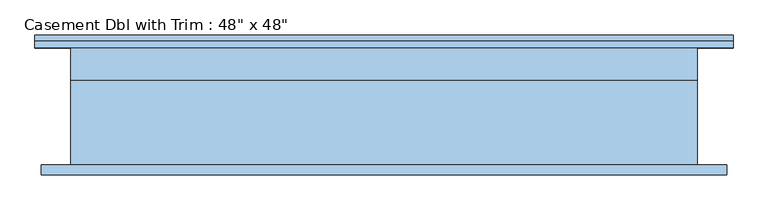
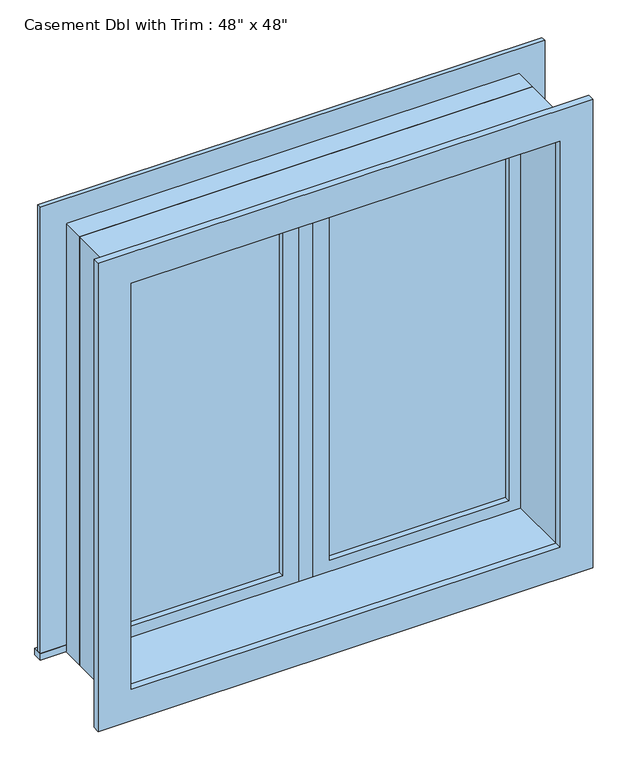
"""IFC4 building model written with IfcOpenShell, lengths in millimetres: window geometry."""

from ifc_helpers import new_model, si_unit, frame, origin, place, context, project, spatial, polyline, outline, extrude, source, transform, mapped, element, save


def window_8af0dca1(model_context):
    return source(origin(), model_context, "Body", "SweptSolid", [
        extrude(outline(polyline([(63.5, 98.425), (546.1, 98.425), (546.1, 85.725), (63.5, 85.725), (63.5, 98.425)])), frame((0.0, 0.0, 825.5), z_axis=(0.0, 0.0, 1.0), x_axis=(1.0, 0.0, 0.0)), (0.0, 0.0, 1.0), 1092.2),
        extrude(outline(polyline([(1962.15, 19.05), (781.05, 19.05), (781.05, 590.55), (1962.15, 590.55), (1962.15, 19.05)]), holes=[polyline([(1917.7, 63.5), (1917.7, 546.1), (825.5, 546.1), (825.5, 63.5), (1917.7, 63.5)])]), frame((0.0, 69.85, 0.0), z_axis=(0.0, 1.0, 0.0), x_axis=(0.0, 0.0, 1.0)), (0.0, 0.0, 1.0), 44.45),
        extrude(outline(polyline([(19.05, 69.85), (-19.05, 69.85), (-19.05, 133.35), (19.05, 133.35), (19.05, 69.85)])), frame((0.0, 0.0, 781.05), z_axis=(0.0, 0.0, 1.0), x_axis=(1.0, 0.0, 0.0)), (0.0, 0.0, 1.0), 1181.1),
        extrude(outline(polyline([(-679.45, 158.75), (679.45, 158.75), (679.45, 133.35), (-679.45, 133.35), (-679.45, 158.75)])), frame((0.0, 0.0, 762.0), z_axis=(0.0, 0.0, 1.0), x_axis=(1.0, 0.0, 0.0)), (0.0, 0.0, 1.0), 19.05),
        extrude(outline(polyline([(1962.15, -590.55), (1962.15, 590.55), (781.05, 590.55), (781.05, 679.45), (2051.05, 679.45), (2051.05, -679.45), (781.05, -679.45), (781.05, -590.55), (1962.15, -590.55)])), frame((0.0, 133.35, 0.0), z_axis=(0.0, 1.0, 0.0), x_axis=(0.0, 0.0, 1.0)), (0.0, 0.0, 1.0), 12.7),
        extrude(outline(polyline([(2038.35, 666.75), (2038.35, -666.75), (704.85, -666.75), (704.85, 666.75), (2038.35, 666.75)]), holes=[polyline([(1949.45, 577.85), (793.75, 577.85), (793.75, -577.85), (1949.45, -577.85), (1949.45, 577.85)])]), frame((0.0, -114.3, 0.0), z_axis=(0.0, 1.0, 0.0), x_axis=(0.0, 0.0, 1.0)), (0.0, 0.0, 1.0), 19.05),
        extrude(outline(polyline([(-63.5, 85.725), (-546.1, 85.725), (-546.1, 98.425), (-63.5, 98.425), (-63.5, 85.725)])), frame((0.0, 0.0, 825.5), z_axis=(0.0, 0.0, 1.0), x_axis=(1.0, 0.0, 0.0)), (0.0, 0.0, 1.0), 1092.2),
        extrude(outline(polyline([(1962.15, -590.55), (781.05, -590.55), (781.05, -19.05), (1962.15, -19.05), (1962.15, -590.55)]), holes=[polyline([(1917.7, -546.1), (1917.7, -63.5), (825.5, -63.5), (825.5, -546.1), (1917.7, -546.1)])]), frame((0.0, 69.85, 0.0), z_axis=(0.0, 1.0, 0.0), x_axis=(0.0, 0.0, 1.0)), (0.0, 0.0, 1.0), 44.45),
        extrude(outline(polyline([(1981.2, -609.6), (762.0, -609.6), (762.0, 609.6), (1981.2, 609.6), (1981.2, -609.6)]), holes=[polyline([(1949.45, -577.85), (1949.45, 577.85), (793.75, 577.85), (793.75, -577.85), (1949.45, -577.85)])]), frame((0.0, -95.25, 0.0), z_axis=(0.0, 1.0, 0.0), x_axis=(0.0, 0.0, 1.0)), (0.0, 0.0, 1.0), 165.1),
        extrude(outline(polyline([(1981.2, 609.6), (1981.2, -609.6), (762.0, -609.6), (762.0, 609.6), (1981.2, 609.6)]), holes=[polyline([(1962.15, 590.55), (781.05, 590.55), (781.05, -590.55), (1962.15, -590.55), (1962.15, 590.55)])]), frame((0.0, 69.85, 0.0), z_axis=(0.0, 1.0, 0.0), x_axis=(0.0, 0.0, 1.0)), (0.0, 0.0, 1.0), 63.5),
    ])


if __name__ == "__main__":
    model = new_model("IFC4")
    model_context = context("Model", 3, world=origin())
    ifc_project = project(units=[si_unit("LENGTHUNIT", "METRE", prefix="MILLI")], contexts=[model_context])
    site = spatial("IfcSite", under=ifc_project)
    building = spatial("IfcBuilding", under=site)
    placement = place(None, origin())
    window_shape = window_8af0dca1(model_context)
    element("IfcWindow", 1, ObjectType="Casement Dbl with Trim : 48\" x 48\"", at=placement, inside=building, context=model_context, shape_type="MappedRepresentation", body=[
        mapped(window_shape, transform((0.0, 0.0, 0.0), x_axis=(1.0, 0.0, 0.0), y_axis=(0.0, 1.0, 0.0), z_axis=(0.0, 0.0, 1.0))),
    ])
    save(model, "model.ifc")

# Revit data of these elements
# Type "Casement Dbl with Trim : 48\" x 48\""
#   Type Mark = "10"
#   Construction Type Id = "GSP4R"
#   Assembly Code = "B2020100"
#   Analytic Construction = "1/8 in Pilkington single glazing"
#   Visual Light Transmittance = 0.9
#   Solar Heat Gain Coefficient = 0.78
#   Heat Transfer Coefficient (U) = 0.6496 BTU/(h·ft²·°F)
#   Height = 4' - 0"
#   Default Sill Height = 2' - 6"
#   Trim Projection - Ext. = 0' - 0 1/2"
#   Trim Projection - Int. = 0' - 0 3/4"
#   Trim Width - Exterior = 0' - 3 1/2"
#   Trim Width - Interior = 0' - 3 1/2"
#   Width = 4' - 0"
#   Window Inset = 0' - 0 3/4"
#   Define Thermal Properties by = 1
#   Glass Pane Material = Glass
#   Sash Material = Sash
#   Trim Exterior Material = Trim
#   Trim Interior Material = Trim
#   Wall Closure = (empty or 0)
# Element 1 (IfcWindow, "Casement Dbl with Trim : 48\" x 48\"")
#   Materials on its faces: "Sash", "Trim", "Glass"
# Materials
#   "Glass": class "Glass", colour RGB 0 128 192, transparency 0.75, Description = "Soda Lime Glass", Cost = 0
#   "Sash": class "Wood", colour RGB 224 178 126, transparency 0
#   "Trim": class "Wood", colour RGB 224 178 126, transparency 0
